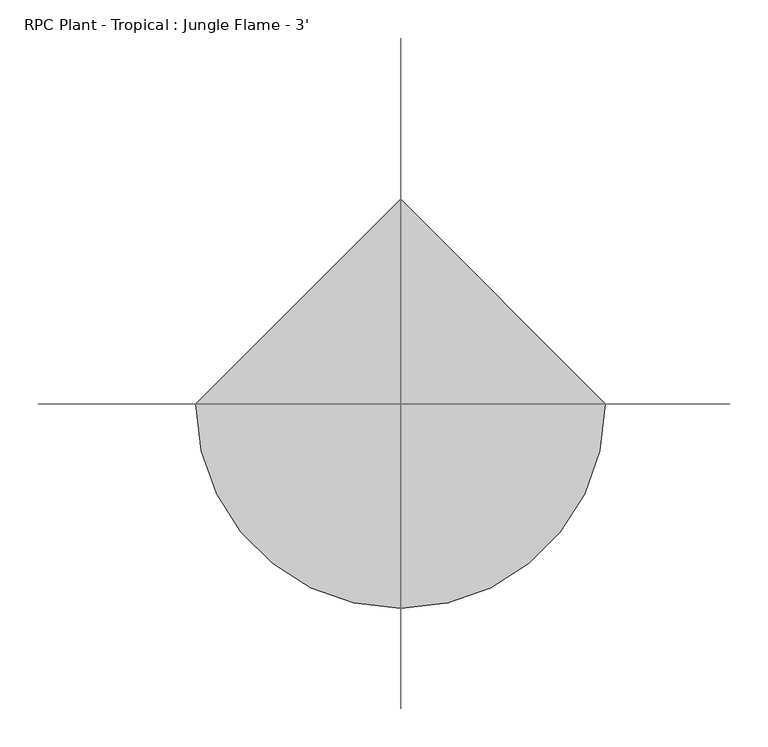
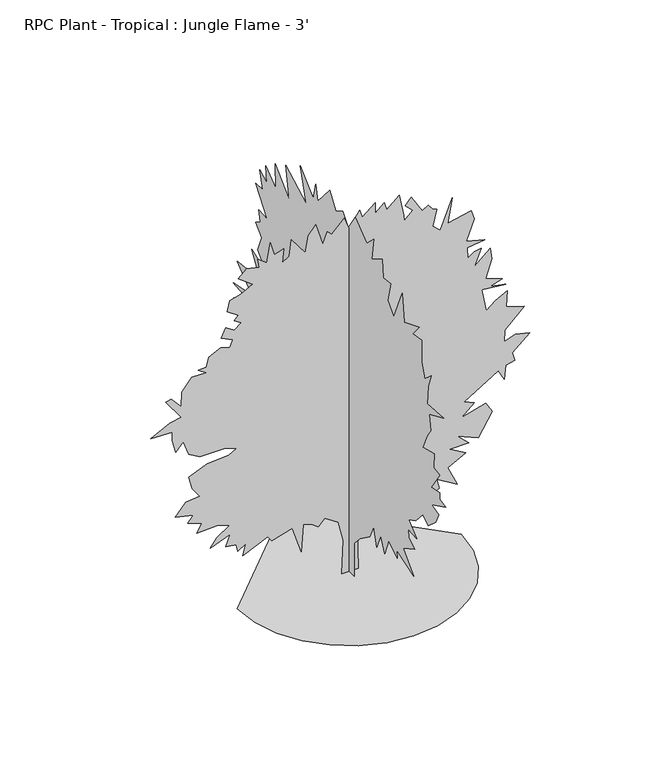
"""IFC4 building model written with IfcOpenShell, lengths in millimetres: geographic element geometry, RPC Plant - Tropical : Jungle Flame - 3'."""

from ifc_helpers import new_model, si_unit, origin, place, context, project, spatial, triangles, source, transform, mapped, element, save


def rpc_plant_tropical_jungle_flame_3_9c4808c2(model_context):
    return source(origin(), model_context, "Body", "Tessellation", [
        triangles([(-268.0952273, 0.0, 4.64e-05), (-261.0086141, -61.4296216, 4.64e-05), (-240.8232365, -117.8430704, 4.64e-05), (-209.155511, -167.6236892, 4.64e-05), (-167.6236892, -209.1557472, 4.64e-05), (-117.8430704, -240.8232365, 4.64e-05), (-61.4296216, -261.0086141, 4.64e-05), (1.17e-05, -268.0952273, 4.64e-05), (61.4296216, -261.0086141, 4.64e-05), (117.8430704, -240.8232365, 4.64e-05), (167.6236892, -209.155511, 4.64e-05), (209.1557472, -167.6236892, 4.64e-05), (240.8232365, -117.8430704, 4.64e-05), (261.0086141, -61.4296216, 4.64e-05), (268.0952273, 2.34e-05, 4.64e-05), (-3.52e-05, 268.0952273, 4.64e-05), (-1.48e-05, -20.1101483, 4.49e-05), (-1.23e-05, -20.1680527, 84.1033148), (-1.26e-05, -43.4307974, 109.1553558), (-1.36e-05, -84.5877148, 139.5758464), (-1.33e-05, -102.4820622, 175.3643141), (-1.52e-05, -115.0079782, 130.6286726), (-1.47e-05, -131.1128455, 169.9961098), (-1.65e-05, -147.2177128, 134.2074059), (-1.6e-05, -163.3225891, 177.1537943), (-1.83e-05, -199.111284, 153.8912426), (-1.76e-05, -197.3218038, 173.5750701), (-2.14e-05, -267.1099495, 150.3122731), (-1.81e-05, -224.163334, 195.0481417), (-1.95e-05, -270.6875473, 220.1001918), (-1.79e-05, -245.6375502, 234.4155789), (-1.73e-05, -243.8476158, 254.100333), (-1.89e-05, -279.6349481, 252.3103987), (-1.66e-05, -247.4252136, 280.9402645), (-1.75e-05, -276.0573685, 295.2574684), (-1.78e-05, -304.6872162, 327.4672211), (-1.92e-05, -327.9495681, 314.9399334), (-1.98e-05, -358.3716574, 341.782154), (-1.95e-05, -370.8966559, 368.6220855), (-1.8e-05, -342.2667901, 375.7818229), (-1.97e-05, -399.5287745, 404.4116887), (-1.85e-05, -374.4765246, 409.7792027), (-1.8e-05, -374.4765246, 425.8840699), (-1.67e-05, -340.4768558, 418.7266216), (-1.67e-05, -374.4765246, 470.6210921), (-1.54e-05, -349.4242384, 474.1987081), (-1.44e-05, -351.2141727, 509.9883113), (-1.27e-05, -304.6872162, 499.250958), (-1.23e-05, -322.5820178, 538.6181771), (-1.23e-05, -336.8969507, 560.0928474), (-1.09e-05, -331.5294368, 597.6701323), (-1.28e-05, -390.5813919, 624.5123165), (-9.9e-06, -322.5820178, 619.1448389), (-8.7e-06, -327.9495681, 667.4594044), (-8.2e-06, -338.6868851, 699.6691389), (-7.7e-06, -311.8447008, 676.4045706), (-6.1e-06, -299.3197022, 710.4042395), (-4.5e-06, -299.3197022, 765.8762896), (-3.1e-06, -263.5300808, 760.5087393), (-3.3e-06, -290.3722833, 792.7184738), (-1.2e-06, -227.7422944, 767.6662239), (1.2e-06, -218.7951116, 835.6655617), (3e-07, -184.7958969, 755.1412617), (2.2e-06, -159.7438468, 781.9811932), (3.2e-06, -172.2697537, 832.085693), (4.4e-06, -141.8494994, 828.5081497), (5.9e-06, -136.4810589, 871.4529121), (7.1e-06, -93.5348885, 846.4006622), (8.4e-06, -100.692582, 900.0851034), (8.9e-06, -72.0615762, 873.2428465), (1.21e-05, -25.5364477, 910.8201313), (1.2e-05, 3.0945581, 866.0853619), (1.39e-05, 26.3571235, 894.7152277), (1.47e-05, 54.9881316, 878.6103968), (1.69e-05, 80.0401726, 914.4), (1.74e-05, 130.1442636, 857.1380156), (1.89e-05, 139.0914373, 894.7152277), (1.81e-05, 149.8281003, 851.7704653), (2.2e-05, 203.5109246, 901.8750378), (1.85e-05, 178.4588745, 821.3506651), (2.37e-05, 262.5630977, 867.8752962), (2.07e-05, 248.2458757, 789.1409306), (2.49e-05, 305.5079146, 844.6129807), (2.3e-05, 303.7202512, 783.7711275), (2.58e-05, 344.8750975, 815.980862), (2.44e-05, 341.2975179, 774.8237085), (2.62e-05, 369.9273837, 790.9285395), (2.43e-05, 357.4023851, 747.983777), (2.56e-05, 387.8221853, 746.1938427), (2.16e-05, 339.5075835, 683.564308), (2.32e-05, 373.5072524, 687.1418512), (2.22e-05, 368.1397385, 660.299667), (2.27e-05, 387.8221853, 647.7747047), (2.08e-05, 362.7698991, 622.7223822), (2.04e-05, 378.8747663, 583.3551993), (1.77e-05, 343.0874522, 547.5655961), (2.11e-05, 403.9270526, 569.0402664), (1.71e-05, 360.9799647, 499.250958), (1.89e-05, 393.1896993, 511.7782456), (2.17e-05, 462.9790077, 502.830863), (1.77e-05, 403.9270526, 454.5162249), (2.05e-05, 479.083875, 438.4113576), (1.67e-05, 396.7696043, 431.2539093), (1.57e-05, 387.8221853, 411.569137), (1.94e-05, 477.2939406, 402.6217544), (1.5e-05, 394.97967, 377.5694681), (1.44e-05, 411.0845372, 332.834735), (1.36e-05, 368.1397385, 370.4120198), (1.19e-05, 355.6124508, 334.6246694), (1.33e-05, 398.5595387, 314.9399334), (1.21e-05, 400.349473, 271.9928455), (8.7e-06, 341.2975179, 248.7305118), (1.01e-05, 384.2446057, 229.0480649), (4.9e-06, 291.1929636, 195.0481417), (6.5e-06, 341.2975179, 175.3643141), (6.7e-06, 369.9273837, 135.996886), (4.2e-06, 294.7728504, 166.4173675), (2.6e-06, 289.4030292, 121.6814898), (2.3e-06, 258.983229, 157.4702029), (0.0, 239.300764, 107.3661027), (1.6e-06, 241.0884092, 159.2594469), (1.2e-06, 228.5629746, 164.6278873), (-1.1e-06, 203.5109246, 127.0497123), (-2e-07, 205.3004047, 153.8912426), (-1.9e-06, 162.3540072, 159.2594469), (-2.4e-06, 167.7222116, 135.996886), (-3e-06, 139.0914373, 157.4702029), (-5.5e-06, 130.1442636, 89.4717553), (-5.5e-06, 74.6719592, 171.78559), (-6.4e-06, 62.1458251, 161.048927), (-7.4e-06, 37.0937796, 164.6278873), (-7.6e-06, 51.4093984, 134.2074059), (-8.5e-06, 15.6205809, 157.4702029), (-1.29e-05, 22.7783675, 4.61e-05), (-17.334692, 5.3e-05, 1.7e-06), (-13.7758477, 4.79e-05, 83.6317139), (-26.2316224, 4.54e-05, 133.4546266), (-58.2607652, 4.56e-05, 154.8074657), (-74.27534, 4.72e-05, 138.7928909), (-90.2899103, 4.72e-05, 151.2486168), (-109.863334, 4.77e-05, 156.5868811), (-115.2013712, 5.19e-05, 90.7491664), (-136.5542103, 4.89e-05, 156.5868811), (-184.5979257, 5.18e-05, 142.3517307), (-195.2742362, 5.15e-05, 156.5868811), (-253.9951796, 5.57e-05, 128.1165803), (-246.8765734, 5.37e-05, 156.5868811), (-266.4493067, 5.53e-05, 144.1311552), (-270.0086098, 5.44e-05, 161.9249273), (-294.9214242, 5.53e-05, 165.4837762), (-284.2435331, 5.31e-05, 193.954077), (-332.2884021, 5.64e-05, 174.3808894), (-316.2726645, 5.44e-05, 195.7334923), (-286.024311, 5.18e-05, 217.0863314), (-316.2726645, 5.26e-05, 225.9832084), (-364.3175517, 5.48e-05, 224.203793), (-351.8611173, 5.31e-05, 243.7767626), (-385.6687921, 5.38e-05, 256.2331607), (-373.2146467, 5.23e-05, 272.2465909), (-415.9194165, 5.36e-05, 282.9245002), (-391.0088731, 5.08e-05, 311.3943649), (-357.1989455, 4.91e-05, 314.953668), (-374.9931719, 4.84e-05, 339.8641751), (-383.8902669, 4.69e-05, 371.8933248), (-339.4047192, 4.38e-05, 391.4660763), (-287.8028362, 4.13e-05, 395.0253794), (-268.2301028, 3.98e-05, 405.7032887), (-300.2592343, 4.07e-05, 414.5980946), (-357.1989455, 4.32e-05, 414.5980946), (-383.8902669, 4.34e-05, 430.6138321), (-396.346665, 4.18e-05, 466.2022848), (-414.1408914, 4.37e-05, 446.6272442), (-423.0357336, 4.22e-05, 478.6563938), (-423.0357336, 4.09e-05, 500.0099233), (-474.6398875, 4.31e-05, 501.7884121), (-428.3758146, 3.97e-05, 524.9227558), (-401.6844933, 3.82e-05, 530.2605477), (-439.0514348, 3.68e-05, 581.8624489), (-424.8165115, 3.6e-05, 583.6409377), (-401.6844933, 3.66e-05, 556.9519054), (-399.903679, 3.44e-05, 592.5380691), (-376.7716607, 3.16e-05, 622.7887299), (-341.1854971, 3.02e-05, 621.0078793), (-360.7582486, 3.02e-05, 635.2450916), (-341.1854971, 2.93e-05, 635.2450916), (-335.8454161, 2.77e-05, 658.3771099), (-307.3755695, 2.56e-05, 672.6120695), (-286.024311, 2.51e-05, 665.4934633), (-278.905723, 2.37e-05, 683.2876534), (-305.5970444, 2.41e-05, 695.7440878), (-294.9214242, 2.23e-05, 718.8761061), (-275.3464199, 2.22e-05, 706.4197443), (-257.5521935, 2.07e-05, 718.8761061), (-275.3464199, 2.08e-05, 729.5517626), (-264.6707997, 1.97e-05, 740.2273464), (-291.3621211, 1.98e-05, 758.0216091), (-286.024311, 1.8e-05, 784.7129305), (-259.3329896, 1.64e-05, 791.8315367), (-230.8631431, 1.43e-05, 806.0664963), (-264.6707997, 1.42e-05, 832.7578176), (-245.0980664, 1.23e-05, 850.5520077), (-214.8476599, 1.14e-05, 843.4334015), (-218.4062726, 1.03e-05, 864.7869673), (-197.0536516, 1.03e-05, 848.7712297), (-188.1565384, 7e-06, 896.8161169), (-179.2596614, 8.7e-06, 863.0061167), (-156.1274069, 7.2e-06, 870.1247229), (-159.6862377, 9.4e-06, 836.3147953), (-143.6716719, 8.1e-06, 846.9927046), (-138.3334077, 5.5e-06, 886.1382076), (-104.5250607, 6.7e-06, 841.6548763), (-97.407372, 3.9e-06, 882.5811573), (-79.6133818, 1.9e-06, 903.9323977), (-63.599034, 4.4e-06, 848.7712297), (-52.922501, 2.3e-06, 877.2410763), (-42.246195, 2.5e-06, 866.5654198), (-11.9964482, -7e-07, 896.8161169), (-1.3200484, 6e-07, 868.3439449), (25.3709418, -2.7e-06, 903.9323977), (30.7089813, -1.8e-06, 884.3596825), (62.7381264, -4.7e-06, 909.2702259), (62.7381264, -3.1e-06, 882.5811573), (84.09097, -5.2e-06, 902.1538725), (89.4290072, -4.3e-06, 882.5811573), (119.6787324, -7.2e-06, 909.2702259), (130.3552609, -4.4e-06, 854.109058), (132.1346854, -3.6e-06, 839.8740984), (151.7078729, -5.6e-06, 859.449139), (133.9138827, -5.9e-06, 877.2410763), (148.1492602, -7.5e-06, 893.2568138), (174.8401455, -6.1e-06, 850.5520077), (189.0752868, -7.2e-06, 859.449139), (197.9721638, -6.9e-06, 846.9927046), (208.6487105, -7e-06, 841.6548763), (199.7515974, -4.3e-06, 802.5071932), (217.5455875, -4.1e-06, 786.4937084), (246.0147437, -9.6e-06, 857.6683611), (235.3391235, -5.5e-06, 797.1693649), (292.2811057, -8.8e-06, 809.6257267), (299.3974228, -7.7e-06, 786.4937084), (279.8246894, -3.9e-06, 736.6703688), (324.3102553, -5.1e-06, 724.2139343), (281.6031964, -2.9e-06, 718.8761061), (283.3839925, -1.4e-06, 692.1847847), (299.3974228, -2.7e-06, 702.8604412), (315.413124, -3.6e-06, 706.4197443), (299.3974228, -5e-07, 665.4934633), (336.7643643, -4.1e-06, 699.3033909), (340.3236674, -2.6e-06, 670.8312916), (326.0887442, 7e-07, 626.348033), (365.2365, -2e-07, 612.1130733), (336.7643643, 1.6e-06, 603.2159783), (374.1313422, 5e-07, 594.318847), (317.1916492, 2.5e-06, 601.4351641), (327.8672693, 5.5e-06, 544.495471), (349.2207988, 3.5e-06, 562.2896974), (377.6906453, 1.4e-06, 576.5246206), (375.9121202, 3.8e-06, 537.3768648), (418.61689, 2.8e-06, 523.1419415), (372.3528171, 7.4e-06, 478.6563938), (370.5743282, 9.2e-06, 450.1865473), (397.2633605, 7.4e-06, 460.8644566), (431.0732881, 6.5e-06, 451.9673615), (390.1470434, 1.04e-05, 416.3789088), (395.4848717, 1.14e-05, 395.0253794), (374.1313422, 1.27e-05, 389.6875511), (370.5743282, 1.48e-05, 355.8799127), (356.339405, 1.39e-05, 382.5689449), (274.4868793, 2.04e-05, 332.747858), (299.3974228, 2e-05, 322.0699851), (267.3682732, 2.3e-05, 295.3786274), (326.0887442, 1.94e-05, 311.3943649), (342.1021926, 2.03e-05, 284.7030072), (308.2945178, 2.51e-05, 229.5418393), (258.47116, 2.6e-05, 250.8953506), (285.1624995, 2.63e-05, 225.9832084), (240.6769336, 2.84e-05, 224.203793), (278.0438933, 2.8e-05, 202.8511901), (235.3391235, 3.13e-05, 179.7189175), (258.47116, 3.32e-05, 129.8957777), (208.6484744, 3.36e-05, 160.1454938), (215.7661722, 3.48e-05, 135.234042), (180.1781736, 3.73e-05, 119.2194762), (146.3698357, 3.69e-05, 149.4691923), (151.7078729, 4.11e-05, 76.5140161), (132.1346854, 3.8e-05, 142.3517307), (82.3115456, 4.26e-05, 101.425477), (91.2084316, 3.97e-05, 144.1311552), (53.8412448, 4.43e-05, 94.3080153), (43.1647072, 4.28e-05, 126.337165), (66.2969707, 3.83e-05, 185.0571818), (34.2678257, 4e-05, 179.7189175), (18.2532304, 4.23e-05, 153.0280322), (21.8120066, 5.13e-05, 0.0)], [[15, 16, 1], [14, 15, 1], [14, 1, 2], [13, 14, 2], [13, 2, 3], [13, 3, 4], [12, 13, 4], [11, 12, 4], [11, 4, 5], [11, 5, 6], [11, 6, 7], [11, 7, 8], [11, 8, 9], [11, 9, 10], [101, 102, 103], [119, 120, 121], [51, 52, 53], [104, 105, 106], [76, 77, 78], [27, 28, 29], [59, 60, 61], [106, 107, 108], [78, 79, 80], [122, 123, 124], [61, 62, 63], [54, 55, 56], [131, 132, 133], [115, 116, 117], [114, 115, 117], [21, 22, 23], [40, 41, 42], [32, 33, 34], [96, 97, 98], [68, 69, 70], [125, 126, 127], [127, 128, 129], [82, 83, 84], [86, 87, 88], [112, 113, 114], [23, 24, 25], [99, 100, 101], [84, 85, 86], [117, 118, 119], [80, 81, 82], [25, 26, 27], [88, 89, 90], [29, 30, 31], [44, 45, 46], [66, 67, 68], [64, 65, 66], [90, 91, 92], [46, 47, 48], [74, 75, 76], [92, 93, 94], [42, 43, 44], [40, 42, 44], [38, 39, 40], [98, 99, 101], [57, 58, 59], [70, 71, 72], [133, 134, 17], [133, 17, 18], [133, 18, 19], [104, 106, 108], [114, 117, 119], [72, 73, 74], [133, 19, 20], [37, 38, 40], [36, 37, 40], [133, 20, 21], [110, 111, 112], [109, 110, 112], [44, 46, 48], [53, 54, 56], [94, 95, 96], [98, 101, 103], [90, 92, 94], [68, 70, 72], [114, 119, 121], [114, 121, 122], [98, 103, 104], [129, 130, 131], [64, 66, 68], [86, 88, 90], [84, 86, 90], [82, 84, 90], [25, 27, 29], [25, 29, 31], [25, 31, 32], [57, 59, 61], [57, 61, 63], [56, 57, 63], [53, 56, 63], [98, 104, 108], [49, 50, 51], [36, 40, 44], [36, 44, 48], [35, 36, 48], [34, 35, 48], [25, 32, 34], [23, 25, 34], [21, 23, 34], [21, 34, 48], [133, 21, 48], [131, 133, 48], [129, 131, 48], [90, 94, 96], [82, 90, 96], [80, 82, 96], [109, 112, 114], [109, 114, 122], [64, 68, 72], [122, 124, 125], [109, 122, 125], [109, 125, 127], [109, 127, 129], [109, 129, 48], [108, 109, 48], [98, 108, 48], [96, 98, 48], [80, 96, 48], [78, 80, 48], [76, 78, 48], [74, 76, 48], [72, 74, 48], [64, 72, 48], [63, 64, 48], [53, 63, 48], [53, 48, 49], [53, 49, 51], [252, 253, 254], [236, 237, 238], [284, 285, 286], [141, 142, 143], [241, 242, 243], [204, 205, 206], [174, 175, 176], [151, 152, 153], [279, 280, 281], [266, 267, 268], [183, 184, 185], [250, 251, 252], [151, 153, 154], [286, 287, 288], [202, 203, 204], [209, 210, 211], [275, 276, 277], [145, 146, 147], [218, 219, 220], [220, 221, 222], [247, 248, 249], [288, 289, 290], [288, 290, 291], [155, 156, 157], [262, 263, 264], [212, 213, 214], [211, 212, 214], [245, 246, 247], [244, 245, 247], [171, 172, 173], [277, 278, 279], [261, 262, 264], [224, 225, 226], [256, 257, 258], [177, 178, 179], [177, 179, 180], [258, 259, 260], [222, 223, 224], [159, 160, 161], [269, 270, 271], [247, 249, 250], [216, 217, 218], [214, 215, 216], [206, 207, 208], [147, 148, 149], [250, 252, 254], [159, 161, 162], [157, 158, 159], [229, 230, 231], [228, 229, 231], [193, 194, 195], [149, 150, 151], [199, 200, 201], [199, 201, 202], [190, 191, 192], [189, 190, 192], [294, 135, 136], [293, 294, 136], [293, 136, 137], [204, 206, 208], [174, 176, 177], [264, 265, 266], [231, 232, 233], [238, 239, 240], [238, 240, 241], [236, 238, 241], [138, 139, 140], [255, 256, 258], [255, 258, 260], [163, 164, 165], [281, 282, 283], [281, 283, 284], [273, 274, 275], [272, 273, 275], [271, 272, 275], [233, 234, 235], [231, 233, 235], [162, 163, 165], [162, 165, 166], [143, 144, 145], [195, 196, 197], [195, 197, 198], [227, 228, 231], [227, 231, 235], [171, 173, 174], [171, 174, 177], [261, 264, 266], [261, 266, 268], [195, 198, 199], [293, 137, 138], [292, 293, 138], [157, 159, 162], [155, 157, 162], [155, 162, 166], [154, 155, 166], [154, 166, 167], [286, 288, 291], [284, 286, 291], [181, 182, 183], [180, 181, 183], [247, 250, 254], [147, 149, 151], [185, 186, 187], [185, 187, 188], [183, 185, 188], [199, 202, 204], [199, 204, 208], [224, 226, 227], [277, 279, 281], [277, 281, 284], [277, 284, 291], [261, 268, 269], [189, 192, 193], [236, 241, 243], [193, 195, 199], [193, 199, 208], [145, 147, 151], [145, 151, 154], [145, 154, 167], [143, 145, 167], [141, 143, 167], [222, 224, 227], [275, 277, 291], [271, 275, 291], [269, 271, 291], [177, 180, 183], [140, 141, 167], [138, 140, 167], [292, 138, 167], [291, 292, 167], [269, 291, 167], [261, 269, 167], [260, 261, 167], [255, 260, 167], [254, 255, 167], [247, 254, 167], [244, 247, 167], [243, 244, 167], [236, 243, 167], [235, 236, 167], [227, 235, 167], [222, 227, 167], [220, 222, 167], [218, 220, 167], [216, 218, 167], [214, 216, 167], [211, 214, 167], [209, 211, 167], [208, 209, 167], [193, 208, 167], [189, 193, 167], [188, 189, 167], [183, 188, 167], [177, 183, 167], [177, 167, 168], [171, 177, 168], [171, 168, 169], [170, 171, 169]], closed=False),
    ])


if __name__ == "__main__":
    model = new_model("IFC4")
    model_context = context("Model", 3, world=origin())
    ifc_project = project(units=[si_unit("LENGTHUNIT", "METRE", prefix="MILLI")], contexts=[model_context])
    site = spatial("IfcSite", under=ifc_project)
    building = spatial("IfcBuilding", under=site)
    placement = place(None, origin())
    rpc_plant_tropical_jungle_flame_3_shape = rpc_plant_tropical_jungle_flame_3_9c4808c2(model_context)
    element("IfcGeographicElement", 1, ObjectType="RPC Plant - Tropical : Jungle Flame - 3'", at=placement, inside=building, context=model_context, shape_type="MappedRepresentation", body=[
        mapped(rpc_plant_tropical_jungle_flame_3_shape, transform((0.0, 0.0, 0.0), x_axis=(1.0, 0.0, 0.0), y_axis=(0.0, 1.0, 0.0), z_axis=(0.0, 0.0, 1.0))),
    ])
    save(model, "model.ifc")

# Revit data of these elements
# Type "RPC Plant - Tropical : Jungle Flame - 3'"
#   built-in parameter 1005198 = "{2, 15},{39, RPC-16-FUVJ-JWG0-MWGK-8000-ST1L-LVER-AU},{1, 0},{1, 0},{2, 35},{1, 8},{5, Color},{1, 0},{1, 0},{3, 0.8},{3, 0.8},{3, 0.8},{1, 8},{7, BBoxMin},{1, 0},{1, 0},{1, 0},{1, 0},{1, 0},{1, 8},{7, BBoxMax},{1, 0},{1, 0},{1, 0},{1, 0},{1, 0},{2, 11},{9, RPCTypeId},{1, 0},{1, 0},{39, RPC-16-FUVJ-JWG0-MWGK-8000-ST1L-LVER-AU},{1, 6},{14, RPCPlantHeight},{1, 0},{1, 0},{1, 3},{2, 11},{7, keyword},{1, 0},{1, 0},{90, :Geometry:RPC:Jungle Flame:ixora macrothyrsa:jungle flame:bush:shrub:plant:flower:tropical},{2, 11},{8, category},{1, 0},{1, 0},{17, :Shrubs [General]},{2, 11},{12, LocalizedUID},{1, 0},{1, 0},{12, Jungle Flame},{2, 14},{6, Height},{1, 0},{1, 0},{1, 3},{1, 2},{16, Cast Reflections},{1, 0},{1, 0},{1, 0},{1, 2},{12, Cast Shadows},{1, 0},{1, 0},{1, 1},{1, 2},{9, Lock View},{1, 0},{1, 0},{1, 0},{1, 4},{5, ViewC},{1, 0},{1, 0},{1, 0},{2, 11},{20, AdvancedUIDefinition},{1, 0},{1, 0},{0, },{2, 11},{10, AssetLibID},{1, 0},{1, 0},{36, 4D3F6E72-3F99-4203-98E9-AF80B3C7A7A4},{2, 11},{10, BaseSchema},{1, 0},{1, 0},{9, RPCSchema},{2, 11},{12, ExchangeGUID},{1, 0},{1, 0},{0, },{1, 2},{6, Hidden},{1, 0},{1, 0},{1, 0},{1, 4},{11, RPCCategory},{1, 0},{1, 0},{1, 0},{2, 11},{8, RPCImage},{1, 0},{1, 0},{0, },{1, 4},{13, SchemaVersion},{1, 0},{1, 0},{1, 4},{2, 11},{12, UIDefinition},{1, 0},{1, 0},{0, },{2, 11},{6, UIName},{1, 0},{1, 0},{39, RPC-16-FUVJ-JWG0-MWGK-8000-ST1L-LVER-AU},{2, 11},{11, VersionGUID},{1, 0},{1, 0},{9, RPCSchema},{2, 11},{9, assettype},{1, 0},{1, 0},{11, RPCGeometry},{2, 11},{11, description},{1, 0},{1, 0},{0, },{2, 11},{9, localname},{1, 0},{1, 0},{3, RPC},{2, 11},{9, localtype},{1, 0},{1, 0},{3, RPC},{1, 4},{8, revision},{1, 0},{1, 0},{1, 1},{2, 11},{9, thumbnail},{1, 0},{1, 0},{0, },{1, 4},{7, version},{1, 0},{1, 0},{1, 1},{1, 2},{20, RPC_Cast Reflections},{1, 0},{1, 0},{1, 1},{1, 2},{16, RPC_Cast Shadows},{1, 0},{1, 0},{1, 1},{1, 2},{13, RPC_Lock View},{1, 0},{1, 0},{1, 0},{1, 4},{9, RPC_ViewC},{1, 0},{1, 0},{1, 0},{21, assetlibrary_base.fbx},{1, 5},"
#   built-in parameter 1005195 = "RPC-16-FUVJ-JWG0-MWGK-8000-ST1L-LVER-AU"
#   Type Comments = "Jungle Flame"
#   Assembly Code = "G2050500"
#   Height = 3' - 0"
#   Default Elevation = 0
